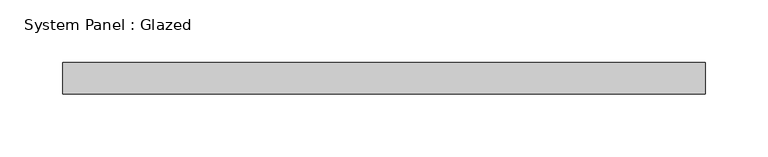
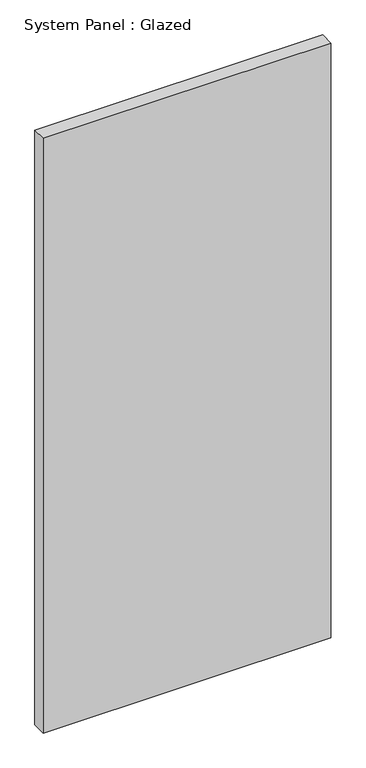
"""IFC4 building model written with IfcOpenShell, lengths in millimetres: plate geometry, System Panel : Glazed."""

from ifc_helpers import new_model, si_unit, origin, origin_with_axes, place, context, project, spatial, polyline, outline, extrude, source, transform, mapped, element, save


def system_panel_glazed_d796fc41(model_context):
    return source(origin(), model_context, "Body", "SweptSolid", [
        extrude(outline(polyline([(257.175, 19.05), (-257.175, 19.05), (-257.175, 44.45), (257.175, 44.45), (257.175, 19.05)])), origin_with_axes(), (0.0, 0.0, 1.0), 1123.95),
    ])


if __name__ == "__main__":
    model = new_model("IFC4")
    model_context = context("Model", 3, world=origin())
    ifc_project = project(units=[si_unit("LENGTHUNIT", "METRE", prefix="MILLI")], contexts=[model_context])
    site = spatial("IfcSite", under=ifc_project)
    building = spatial("IfcBuilding", under=site)
    placement = place(None, origin())
    system_panel_glazed_shape = system_panel_glazed_d796fc41(model_context)
    element("IfcPlate", 1, ObjectType="System Panel : Glazed", at=placement, inside=building, context=model_context, shape_type="MappedRepresentation", body=[
        mapped(system_panel_glazed_shape, transform((0.0, 0.0, 0.0), x_axis=(1.0, 0.0, 0.0), y_axis=(0.0, 1.0, 0.0), z_axis=(0.0, 0.0, 1.0))),
    ])
    save(model, "model.ifc")

# Revit data of these elements
# Type "System Panel : Glazed"
#   Construction Type Id = "GSP4R"
#   Analytic Construction = "1/8 in Pilkington single glazing"
#   Visual Light Transmittance = 0.9
#   Solar Heat Gain Coefficient = 0.86
#   Heat Transfer Coefficient (U) = 1.18115 BTU/(h·ft²·°F)
#   Define Thermal Properties by = 1
# Element 1 (IfcPlate, "System Panel : Glazed")
#   Materials on its faces: "Glass"
# Materials
#   "Glass": class "Glass", colour RGB 0 128 192, transparency 0.75, Description = "Soda Lime Glass", Cost = 0
